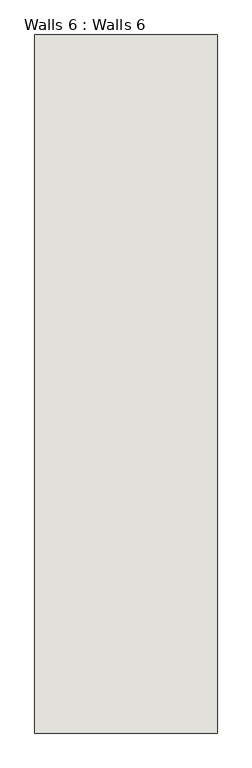
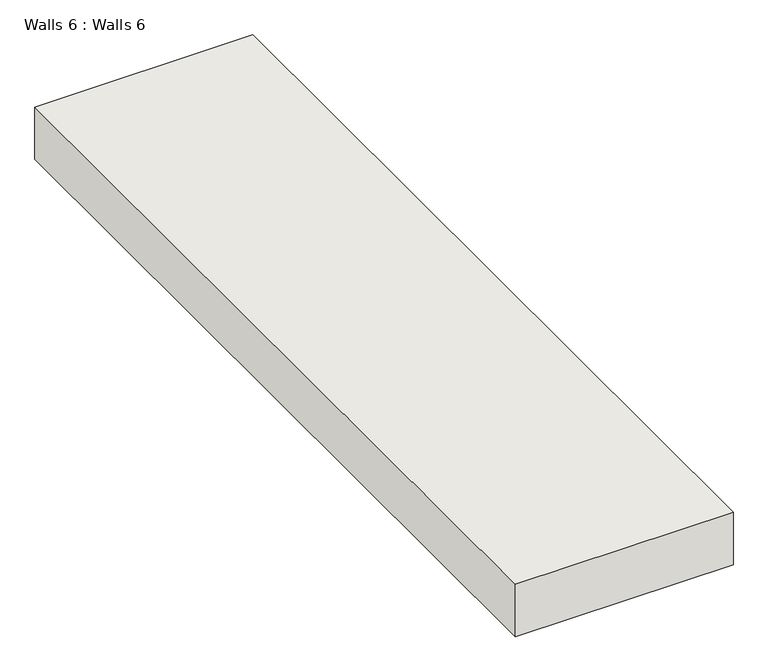
"""IFC4 building model written with IfcOpenShell, lengths in millimetres: wall geometry, Walls 6 : Walls 6."""

from ifc_helpers import new_model, si_unit, frame, origin, place, context, project, spatial, polyline, outline, extrude, source, transform, mapped, element, save


def walls_6_walls_6_3012a6d8(model_context):
    return source(origin(), model_context, "Body", "SweptSolid", [
        extrude(outline(polyline([(-10922.7078307, 11358.0609482), (-10922.7078307, 6786.0609482), (-12118.8440117, 6786.0609482), (-12118.8440117, 11358.0609482), (-10922.7078307, 11358.0609482)])), frame((0.0, 0.0, 10363.2), z_axis=(0.0, 0.0, 1.0), x_axis=(1.0, 0.0, 0.0)), (0.0, 0.0, 1.0), 304.8),
    ])


if __name__ == "__main__":
    model = new_model("IFC4")
    model_context = context("Model", 3, world=origin())
    ifc_project = project(units=[si_unit("LENGTHUNIT", "METRE", prefix="MILLI")], contexts=[model_context])
    site = spatial("IfcSite", under=ifc_project)
    building = spatial("IfcBuilding", under=site)
    placement = place(None, origin())
    walls_6_walls_6_shape = walls_6_walls_6_3012a6d8(model_context)
    element("IfcWall", 1, ObjectType="Walls 6 : Walls 6", at=placement, inside=building, context=model_context, shape_type="MappedRepresentation", body=[
        mapped(walls_6_walls_6_shape, transform((0.0, 0.0, 0.0), x_axis=(1.0, 0.0, 0.0), y_axis=(0.0, 1.0, 0.0), z_axis=(0.0, 0.0, 1.0))),
    ])
    save(model, "model.ifc")

# Revit data of these elements
# Element 1 (IfcWall, "Walls 6 : Walls 6")
#   Materials on its faces: "Default Wall"
# Materials
#   "Default Wall": colour RGB 128 128 128, transparency 0
